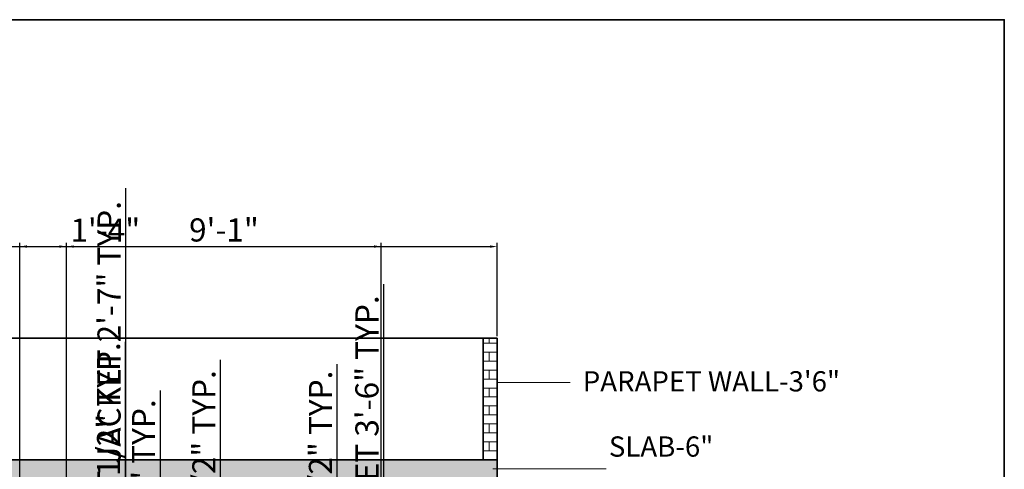
# Model space of a CAD drawing. Units: inches. Extents: x 2257 to 3678, y 834 to 1975.
# Tile 16 of 16: x 3338 to 3678, y 1820 to 1975. Entities that reach past the tile are written whole.
import ezdxf

# ---------------------------------------------------------------- set-up
doc = ezdxf.new("R2010")
doc.units = ezdxf.units.IN
for name, color, linetype, lineweight in [('A-ANNO-DIMS', 2, 'Continuous', 18), ('A-ANNO-TEXT', 7, 'Continuous', 18), ('A-ANNO-TTLB', 7, 'Continuous', 35), ('A-SECT', 7, 'Continuous', 35), ('A-SECT-BRCK-PATT', 252, 'Continuous', 13), ('A-SECT-CONC-PATT', 252, 'Continuous', 13)]:
    doc.layers.add(name, color=color, linetype=linetype, lineweight=lineweight)
doc.styles.get("Standard").update_dxf_attribs({"font": 'arial.ttf'})
doc.dimstyles.new('ISO-25', dxfattribs={"dimtxt": 8, "dimasz": 2.5, "dimexe": 1.25, "dimexo": 0.625, "dimtad": 1, "dimdec": 0, "dimlunit": 3, "dimtxsty": 'Standard', "dimcen": 2.5, "dimadec": 0, "dimazin": 0, "dimtfac": 1, "dimtdec": 0, "dimtmove": 0, "dimatfit": 3, "dimfxl": 1, "dimarcsym": 0})

# ---------------------------------------------------------------- blocks, each defined once
blk = doc.blocks.new('*D85')
at = {"layer": 'A-ANNO-DIMS', "color": 0, "lineweight": -2, "transparency": 16777216}
for p, q in [((3374.21, 1793.13), (3374.21, 1863.53)), ((3376.43, 1793.13), (3372.96, 1793.13)), ((3374.21, 1782.13), (3374.21, 1790.63)), ((3376.43, 1779.63), (3372.96, 1779.63))]:
    blk.add_line(p, q, dxfattribs=at)
at = {"layer": 'A-ANNO-DIMS', "color": 0, "transparency": 16777216}
for points in [[(3373.79, 1790.63), (3374.62, 1790.63), (3374.21, 1793.13)], [(3373.79, 1782.13), (3374.62, 1782.13), (3374.21, 1779.63)]]:
    blk.add_solid(points, dxfattribs=at)
at = {"layer": 'Defpoints', "color": 0, "transparency": 16777216}
for p in [(3374.21, 1793.13), (3377.06, 1793.13), (3377.06, 1779.63)]:
    blk.add_point(p, dxfattribs=at)
at = {"layer": 'A-ANNO-DIMS', "color": 0, "transparency": 16777216, "insert": (3369.44, 1829.58), "char_height": 8, "attachment_point": 5, "rotation": 90}
blk.add_mtext('1\'-1 1/2" TYP.', dxfattribs=at)
blk = doc.blocks.new('*D86')
at = {"layer": 'A-ANNO-DIMS', "color": 0, "lineweight": -2, "transparency": 16777216}
for p, q in [((3374.38, 1776.04), (3374.38, 1916.69)), ((3378.38, 1776.04), (3373.13, 1776.04)), ((3374.38, 1747.73), (3374.38, 1773.54)), ((3378.38, 1745.23), (3373.13, 1745.23))]:
    blk.add_line(p, q, dxfattribs=at)
at = {"layer": 'A-ANNO-DIMS', "color": 0, "transparency": 16777216}
for points in [[(3373.96, 1773.54), (3374.8, 1773.54), (3374.38, 1776.04)], [(3373.96, 1747.73), (3374.8, 1747.73), (3374.38, 1745.23)]]:
    blk.add_solid(points, dxfattribs=at)
at = {"layer": 'Defpoints', "color": 0, "transparency": 16777216}
for p in [(3374.38, 1776.04), (3379, 1776.04), (3379, 1745.23)]:
    blk.add_point(p, dxfattribs=at)
at = {"layer": 'A-ANNO-DIMS', "color": 0, "transparency": 16777216, "insert": (3369.62, 1847.62), "char_height": 8, "attachment_point": 5, "rotation": 90}
blk.add_mtext('SHORT JACKET 2\'-7" TYP.', dxfattribs=at)
blk = doc.blocks.new('*D88')
at = {"layer": 'A-ANNO-DIMS', "color": 0, "lineweight": -2, "transparency": 16777216}
for p, q in [((3386.31, 1728.42), (3386.31, 1846.75)), ((3383.26, 1728.42), (3387.56, 1728.42)), ((3386.31, 1706.41), (3386.31, 1725.92)), ((3383.26, 1703.91), (3387.56, 1703.91))]:
    blk.add_line(p, q, dxfattribs=at)
at = {"layer": 'A-ANNO-DIMS', "color": 0, "transparency": 16777216}
for points in [[(3385.89, 1725.92), (3386.72, 1725.92), (3386.31, 1728.42)], [(3385.89, 1706.41), (3386.72, 1706.41), (3386.31, 1703.91)]]:
    blk.add_solid(points, dxfattribs=at)
at = {"layer": 'Defpoints', "color": 0, "transparency": 16777216}
for p in [(3382.63, 1728.42), (3386.31, 1728.42), (3382.63, 1703.91)]:
    blk.add_point(p, dxfattribs=at)
at = {"layer": 'A-ANNO-DIMS', "color": 0, "transparency": 16777216, "insert": (3381.55, 1788.84), "char_height": 8, "attachment_point": 5, "rotation": 90}
blk.add_mtext('SLACKS 2\'-0 1/2" TYP.', dxfattribs=at)
blk = doc.blocks.new('*D90')
at = {"layer": 'A-ANNO-DIMS', "color": 0, "lineweight": -2, "transparency": 16777216}
for p, q in [((3463.51, 1750.62), (3463.51, 1883.51)), ((3457.86, 1750.62), (3464.76, 1750.62)), ((3463.51, 1711.27), (3463.51, 1748.12)), ((3457.86, 1708.77), (3464.76, 1708.77))]:
    blk.add_line(p, q, dxfattribs=at)
at = {"layer": 'A-ANNO-DIMS', "color": 0, "transparency": 16777216}
for points in [[(3463.09, 1748.12), (3463.92, 1748.12), (3463.51, 1750.62)], [(3463.09, 1711.27), (3463.92, 1711.27), (3463.51, 1708.77)]]:
    blk.add_solid(points, dxfattribs=at)
at = {"layer": 'Defpoints', "color": 0, "transparency": 16777216}
for p in [(3457.23, 1750.62), (3463.51, 1750.62), (3457.23, 1708.77)]:
    blk.add_point(p, dxfattribs=at)
at = {"layer": 'A-ANNO-DIMS', "color": 0, "transparency": 16777216, "insert": (3458.74, 1818.32), "char_height": 8, "attachment_point": 5, "rotation": 90}
blk.add_mtext('LONG JACKET 3\'-6" TYP.', dxfattribs=at)
blk = doc.blocks.new('*D92')
at = {"layer": 'A-ANNO-DIMS', "color": 0, "lineweight": -2, "transparency": 16777216}
for p, q in [((3447.43, 1750.59), (3447.43, 1855.81)), ((3441.81, 1750.59), (3448.68, 1750.59)), ((3447.43, 1711.44), (3447.43, 1748.09)), ((3441.81, 1708.94), (3448.68, 1708.94))]:
    blk.add_line(p, q, dxfattribs=at)
at = {"layer": 'A-ANNO-DIMS', "color": 0, "transparency": 16777216}
for points in [[(3447.01, 1748.09), (3447.85, 1748.09), (3447.43, 1750.59)], [(3447.01, 1711.44), (3447.85, 1711.44), (3447.43, 1708.94)]]:
    blk.add_solid(points, dxfattribs=at)
at = {"layer": 'Defpoints', "color": 0, "transparency": 16777216}
for p in [(3441.18, 1750.59), (3447.43, 1750.59), (3441.18, 1708.94)]:
    blk.add_point(p, dxfattribs=at)
at = {"layer": 'A-ANNO-DIMS', "color": 0, "transparency": 16777216, "insert": (3442.66, 1804.45), "char_height": 8, "attachment_point": 5, "rotation": 90}
blk.add_mtext('COAT 3\'-5 1/2" TYP.', dxfattribs=at)
blk = doc.blocks.new('*D94')
at = {"layer": 'A-ANNO-DIMS', "color": 0, "lineweight": -2, "transparency": 16777216}
for p, q in [((3407.15, 1728.42), (3407.15, 1857.31)), ((3410.23, 1728.42), (3405.9, 1728.42)), ((3407.15, 1706.24), (3407.15, 1725.92)), ((3410.23, 1703.74), (3405.9, 1703.74))]:
    blk.add_line(p, q, dxfattribs=at)
at = {"layer": 'A-ANNO-DIMS', "color": 0, "transparency": 16777216}
for points in [[(3406.73, 1725.92), (3407.57, 1725.92), (3407.15, 1728.42)], [(3406.73, 1706.24), (3407.57, 1706.24), (3407.15, 1703.74)]]:
    blk.add_solid(points, dxfattribs=at)
at = {"layer": 'Defpoints', "color": 0, "transparency": 16777216}
for p in [(3407.15, 1728.42), (3410.85, 1728.42), (3410.85, 1703.74)]:
    blk.add_point(p, dxfattribs=at)
at = {"layer": 'A-ANNO-DIMS', "color": 0, "transparency": 16777216, "insert": (3402.39, 1794.12), "char_height": 8, "attachment_point": 5, "rotation": 90}
blk.add_mtext('SLACKS B 2\'-0 1/2" TYP.', dxfattribs=at)
blk = doc.blocks.new('*D133')
at = {"layer": 'A-ANNO-DIMS', "color": 0, "lineweight": -2, "transparency": 16777216}
for p, q in [((3004.7, 1865.47), (3004.7, 1897.74)), ((3007.2, 1896.49), (3500.2, 1896.49)), ((3502.7, 1865.47), (3502.7, 1897.74))]:
    blk.add_line(p, q, dxfattribs=at)
at = {"layer": 'A-ANNO-DIMS', "color": 0, "transparency": 16777216}
for points in [[(3007.2, 1896.91), (3007.2, 1896.07), (3004.7, 1896.49)], [(3500.2, 1896.91), (3500.2, 1896.07), (3502.7, 1896.49)]]:
    blk.add_solid(points, dxfattribs=at)
at = {"layer": 'Defpoints', "color": 0, "transparency": 16777216}
for p in [(3502.7, 1896.49), (3004.7, 1864.84), (3502.7, 1864.84)]:
    blk.add_point(p, dxfattribs=at)
at = {"layer": 'A-ANNO-DIMS', "color": 0, "transparency": 16777216, "insert": (3253.7, 1901.2), "char_height": 8, "attachment_point": 5}
blk.add_mtext('41\'-6"', dxfattribs=at)
blk = doc.blocks.new('*D138')
at = {"layer": 'A-ANNO-DIMS', "color": 0, "lineweight": -2, "transparency": 16777216}
for p, q in [((3353.91, 1806.08), (3353.91, 1897.74)), ((3356.41, 1896.49), (3460.16, 1896.49)), ((3462.66, 1806.08), (3462.66, 1897.74))]:
    blk.add_line(p, q, dxfattribs=at)
at = {"layer": 'A-ANNO-DIMS', "color": 0, "transparency": 16777216}
for points in [[(3356.41, 1896.91), (3356.41, 1896.07), (3353.91, 1896.49)], [(3460.16, 1896.91), (3460.16, 1896.07), (3462.66, 1896.49)]]:
    blk.add_solid(points, dxfattribs=at)
at = {"layer": 'Defpoints', "color": 0, "transparency": 16777216}
for p in [(3462.66, 1896.49), (3353.91, 1805.46), (3462.66, 1805.46)]:
    blk.add_point(p, dxfattribs=at)
at = {"layer": 'A-ANNO-DIMS', "color": 0, "transparency": 16777216, "insert": (3408.29, 1901.2), "char_height": 8, "attachment_point": 5}
blk.add_mtext('9\'-1"', dxfattribs=at)
blk = doc.blocks.new('*D140')
at = {"layer": 'A-ANNO-DIMS', "color": 0, "lineweight": -2, "transparency": 16777216}
for p, q in [((3337.7, 1697.47), (3337.7, 1897.74)), ((3340.2, 1896.49), (3351.41, 1896.49)), ((3353.91, 1697.33), (3353.91, 1897.74)), ((3353.91, 1896.49), (3378.17, 1896.49))]:
    blk.add_line(p, q, dxfattribs=at)
at = {"layer": 'A-ANNO-DIMS', "color": 0, "transparency": 16777216}
for points in [[(3340.2, 1896.91), (3340.2, 1896.07), (3337.7, 1896.49)], [(3351.41, 1896.91), (3351.41, 1896.07), (3353.91, 1896.49)]]:
    blk.add_solid(points, dxfattribs=at)
at = {"layer": 'Defpoints', "color": 0, "transparency": 16777216}
for p in [(3353.91, 1896.49), (3337.7, 1696.84), (3353.91, 1696.7)]:
    blk.add_point(p, dxfattribs=at)
at = {"layer": 'A-ANNO-DIMS', "color": 0, "transparency": 16777216, "insert": (3367.29, 1901.13), "char_height": 8, "attachment_point": 5}
blk.add_mtext('1\'-4"', dxfattribs=at)

msp = doc.modelspace()

# ---------------------------------------------------------------- hatches: boundary and pattern name
at = {"layer": 'A-SECT-BRCK-PATT'}
h = msp.add_hatch(dxfattribs=at)
h.set_pattern_fill('BRICK', color=256, scale=0.488189, style=0)
h.paths.add_polyline_path([(3497.84, 1822.84), (3502.7, 1822.84), (3502.7, 1864.84), (3497.84, 1864.84)])
at = {"layer": 'A-SECT-CONC-PATT'}
h = msp.add_hatch(dxfattribs=at)
h.set_pattern_fill('AR-CONC', color=256, scale=0.035, style=0)
h.paths.add_polyline_path([(3004.7, 1816.84), (3502.7, 1816.84), (3502.7, 1822.84), (3004.7, 1822.84)])

# ---------------------------------------------------------------- linework, layer by layer
at = {"layer": 'A-ANNO-TEXT'}
for p, q in [((3502.7, 1849.46), (3527.98, 1849.46)), ((3501.26, 1819.67), (3540.38, 1819.67))]:
    msp.add_line(p, q, dxfattribs=at)
at = {"layer": 'A-ANNO-TTLB'}
msp.add_lwpolyline([(2257.38, 1974.9), (3677.96, 1974.9), (3677.96, 849.42), (2257.38, 849.42)], close=True, dxfattribs=at)
at = {"layer": 'A-SECT'}
for p, q in [((3502.7, 1864.84), (3004.7, 1864.84)), ((3497.84, 1822.84), (3497.84, 1864.84)), ((3502.7, 1864.84), (3502.7, 1678.84)), ((3502.7, 1822.84), (3004.7, 1822.84))]:
    msp.add_line(p, q, dxfattribs=at)

# ---------------------------------------------------------------- texts
at = {"layer": 'A-ANNO-TEXT', "char_height": 7, "attachment_point": 1}
for s, width, insert in [('PARAPET WALL-3\'6"', 121.2767, (3532.29, 1853.42)), ('SLAB-6"', 40.0915, (3541.31, 1830.88))]:
    msp.add_mtext_dynamic_manual_height_columns(s, width=width, gutter_width=12.5, heights=[0], dxfattribs=dict(at, insert=insert))

# ---------------------------------------------------------------- dimensions: what is measured, and where the dimension line sits
at = {"layer": 'A-ANNO-DIMS'}
for base, p1, p2, text, picture, middle in [((3374.38, 1776.04), (3379, 1745.23), (3379, 1776.04), 'SHORT JACKET <> TYP.', '*D86', (3369.62, 1847.62)), ((3463.5083, 1750.6208), (3457.2306, 1708.7697), (3457.2306, 1750.6208), 'LONG JACKET <> TYP.', '*D90', (3458.7414, 1818.3161)), ((3374.21, 1793.13), (3377.06, 1779.63), (3377.06, 1793.13), '<> TYP.', '*D85', (3369.44, 1829.58)), ((3407.15, 1728.42), (3410.85, 1703.74), (3410.85, 1728.42), 'SLACKS B <> TYP.', '*D94', (3402.39, 1794.12)), ((3447.4307, 1750.5944), (3441.1821, 1708.9374), (3441.1821, 1750.5944), 'COAT <> TYP.', '*D92', (3442.6638, 1804.4506)), ((3386.31, 1728.42), (3382.63, 1703.91), (3382.63, 1728.42), 'SLACKS <> TYP.', '*D88', (3381.55, 1788.84))]:
    dim = msp.add_linear_dim(base=base, p1=p1, p2=p2, angle=90, text=text, dimstyle='ISO-25', override={"dimdec": 1, "dimlfac": 1, "dimrnd": 0, "dimzin": 1, "dimdsep": 46, "dimlunit": 4, "dimfrac": 2}, dxfattribs=at)
    dim.commit()
    dim.dimension.update_dxf_attribs({"geometry": picture, "text_midpoint": middle})
for base, p1, p2, picture, middle in [((3502.7, 1896.49), (3004.7, 1864.84), (3502.7, 1864.84), '*D133', (3253.7, 1901.2)), ((3353.91, 1896.49), (3337.7, 1696.84), (3353.91, 1696.7), '*D140', (3367.29, 1901.13)), ((3462.662, 1896.4905), (3353.9086, 1805.4561), (3462.662, 1805.4561), '*D138', (3408.2853, 1901.2001))]:
    dim = msp.add_linear_dim(base=base, p1=p1, p2=p2, dimstyle='ISO-25', override={"dimdec": 1, "dimlfac": 1, "dimrnd": 0, "dimzin": 1, "dimdsep": 46, "dimlunit": 4, "dimfrac": 2}, dxfattribs=at)
    dim.commit()
    dim.dimension.update_dxf_attribs({"geometry": picture, "text_midpoint": middle})

doc.saveas('drawing.dxf')
